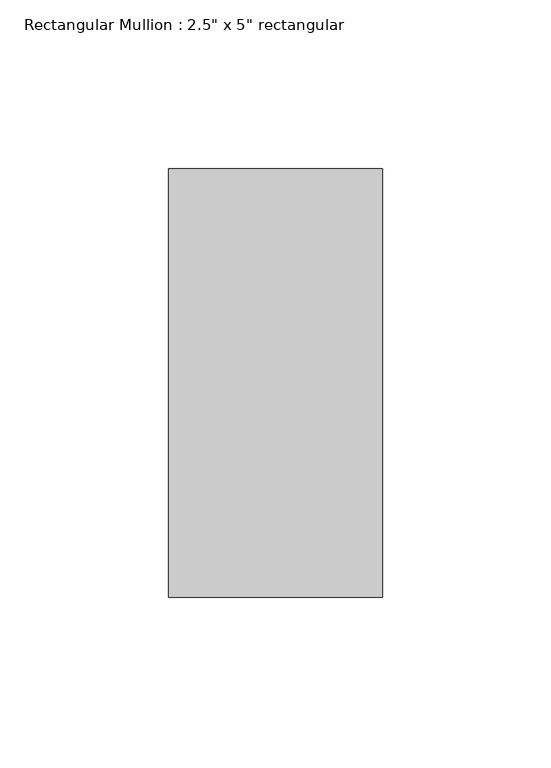
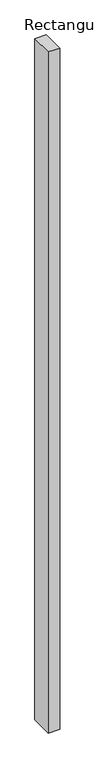
"""IFC4 building model written with IfcOpenShell, lengths in millimetres: member geometry."""

from ifc_helpers import new_model, si_unit, frame, origin, place, context, project, spatial, polyline, outline, extrude, source, transform, mapped, element, save


def member_ec2bec36(model_context):
    return source(origin(), model_context, "Body", "SweptSolid", [
        extrude(outline(polyline([(0.0, 63.5), (0.0, -63.5), (-63.5, -63.5), (-63.5, 63.5), (0.0, 63.5)])), frame((0.0, 0.0, -3987.8), z_axis=(0.0, 0.0, 1.0), x_axis=(1.0, 0.0, 0.0)), (0.0, 0.0, 1.0), 3987.8),
    ])


if __name__ == "__main__":
    model = new_model("IFC4")
    model_context = context("Model", 3, world=origin())
    ifc_project = project(units=[si_unit("LENGTHUNIT", "METRE", prefix="MILLI")], contexts=[model_context])
    site = spatial("IfcSite", under=ifc_project)
    building = spatial("IfcBuilding", under=site)
    placement = place(None, origin())
    member_shape = member_ec2bec36(model_context)
    element("IfcMember", 1, ObjectType="Rectangular Mullion : 2.5\" x 5\" rectangular", at=placement, inside=building, context=model_context, shape_type="MappedRepresentation", body=[
        mapped(member_shape, transform((0.0, 0.0, 0.0), x_axis=(1.0, 0.0, 0.0), y_axis=(0.0, 1.0, 0.0), z_axis=(0.0, 0.0, 1.0))),
    ])
    save(model, "model.ifc")

# Revit data of these elements
# Type "Rectangular Mullion : 2.5\" x 5\" rectangular"
#   built-in parameter 1007304 = 0.416667 (stored number, unit not read)
#   built-in parameter 1007301 = 0.104167 (stored number, unit not read)
#   built-in parameter 1007300 = 0.104167 (stored number, unit not read)
# Element 1 (IfcMember, "Rectangular Mullion : 2.5\" x 5\" rectangular")
#   Materials on its faces: "Iron, Ductile"
# Materials
#   "Iron, Ductile": class "Metal", colour RGB 0 0 0, transparency 0, Description = "Ductile cast iron", Cost = 0
